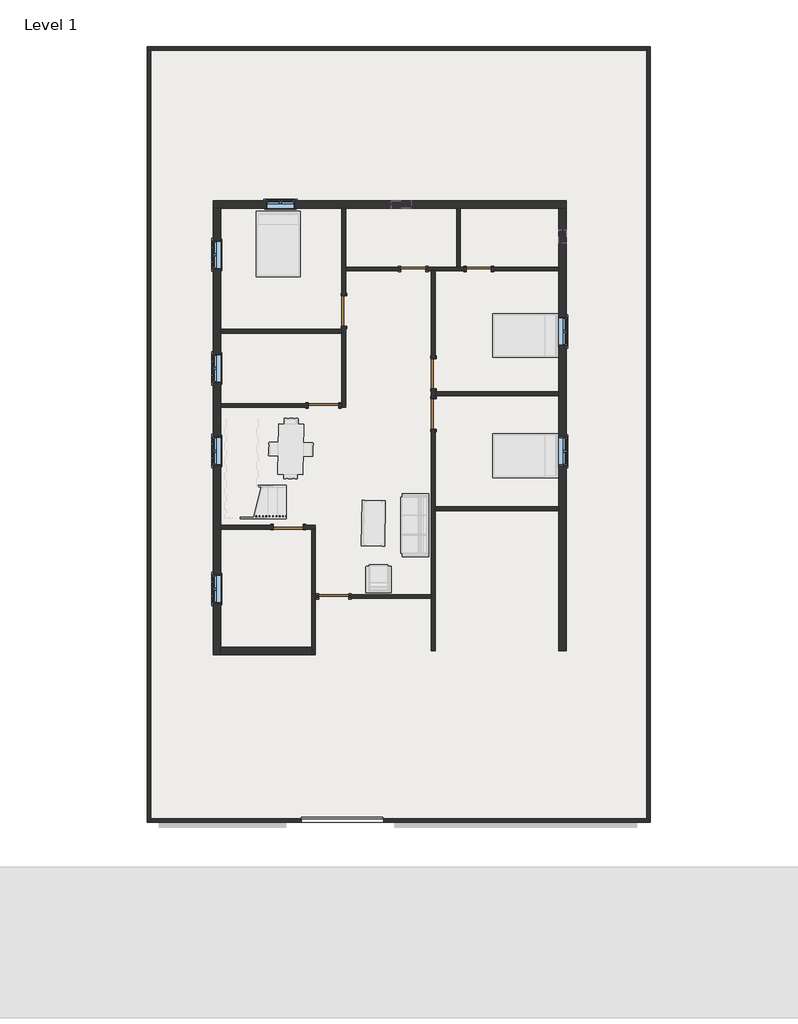
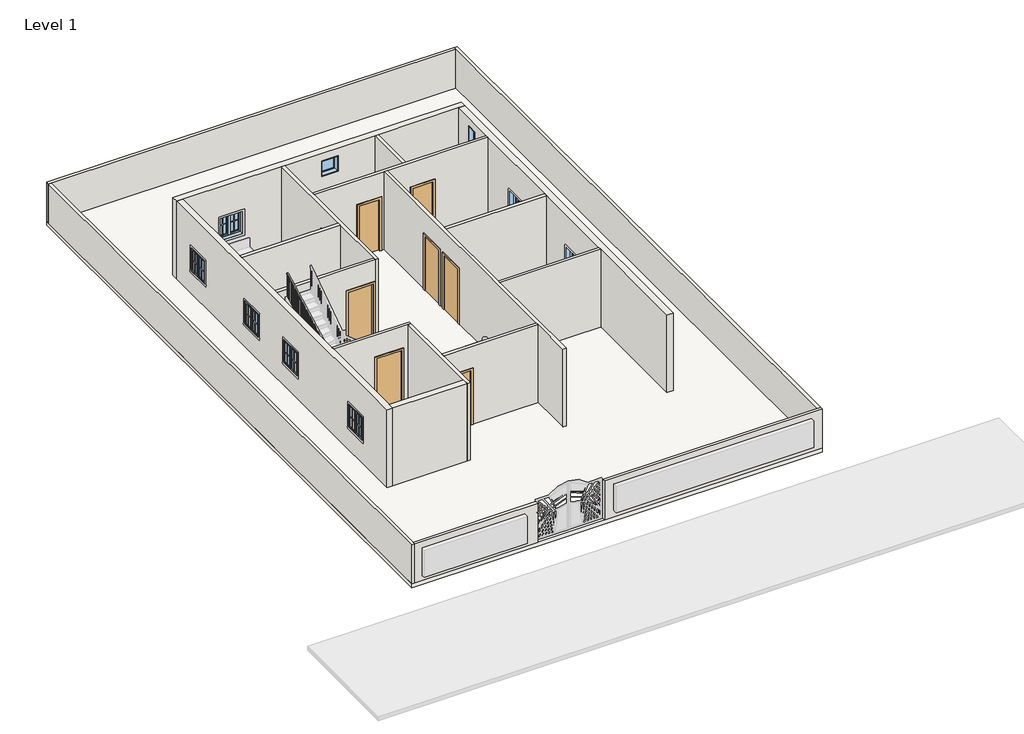
# One storey, part 1 of 2: 20 walls, 9 windows, 8 doors, 1 railing, 1 slab.
# Revit data of these elements (continued)
# Element 39 (IfcWindow, "Window-Casement-Double : 34\" x 36\"") (continued)
#   Exterior Wall Closure = 0' - 1 1/4"
#   Interior Trim Visibility = yes
#   Exterior Trim Visibility = yes
#   Phase Created = New Construction
#   Materials on its faces: "Wood - Stained", "Glass", "Clad - White"
# Materials
#   "Door - Panel": class "Wood", colour RGB 210 159 95, transparency 0, Cost = 0
#   "Door - Frame": colour RGB 118 70 51, transparency 0, Cost = 0
#   "Glass": class "Glass", colour RGB 0 128 192, transparency 0.75, Description = "Soda Lime Glass", Cost = 0
#   "Sash": class "Wood", colour RGB 224 178 126, transparency 0, Cost = 0
#   "Wood - Stained": class "Wood", colour RGB 224 178 126, transparency 0, Cost = 0
#   "Clad - White": class "Wood", colour RGB 242 242 238, transparency 0, Cost = 0
#   "Default Floor": colour RGB 128 128 128, transparency 0, Cost = 0
#   "legs": colour RGB 90 73 37, transparency 0, Cost = 0
#   "Default Wall": colour RGB 128 128 128, transparency 0, Cost = 0
#   "Oak Flooring": class "Wood", colour RGB 216 169 114, transparency 0, Description = "Quercus Rubra", Cost = 0
